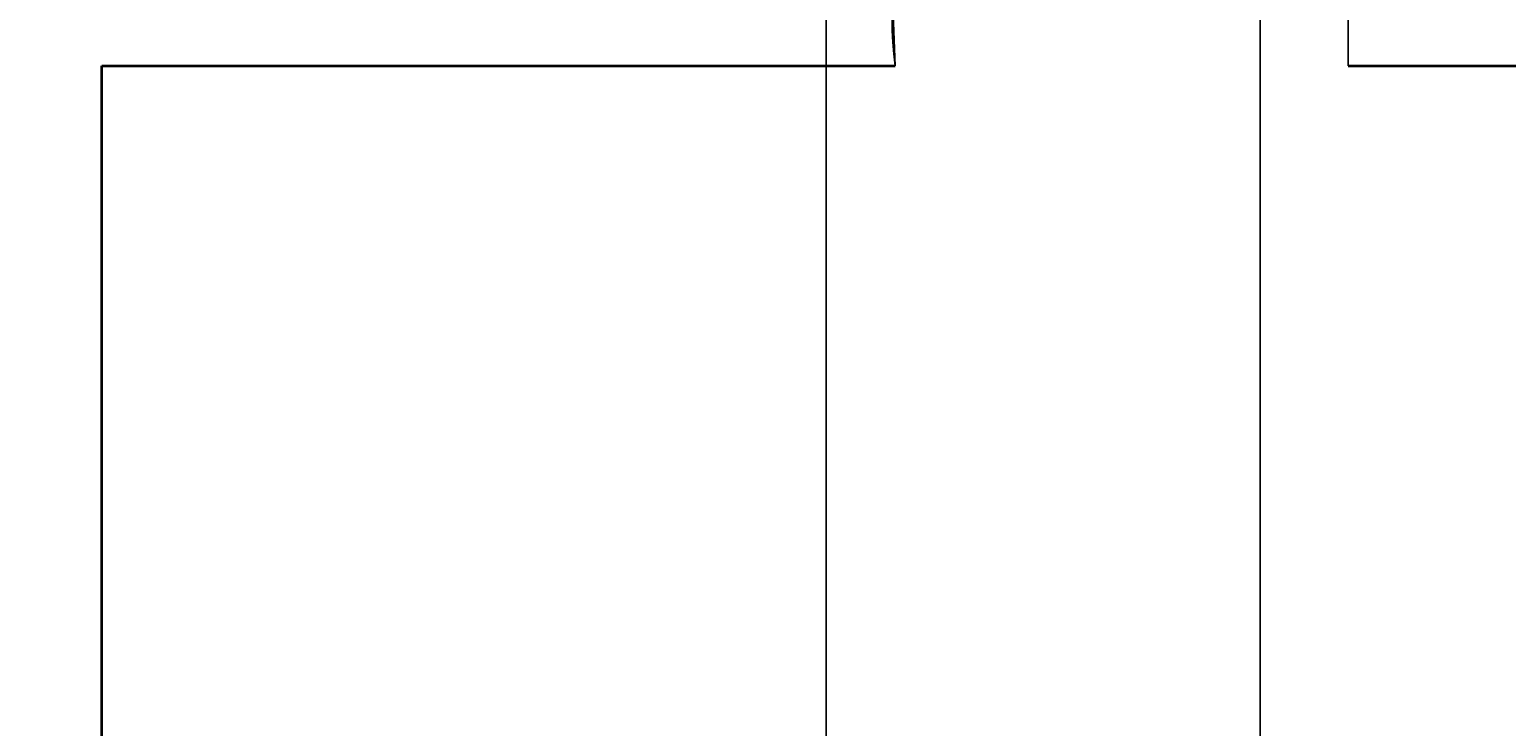
# Model space of a CAD drawing. Units: inches. Extents: x -61 to 1599, y -1316 to 257.
# Tile 111 of 204: x 114 to 236, y -68 to -10. Entities that reach past the tile are written whole.
import ezdxf

# ---------------------------------------------------------------- set-up
doc = ezdxf.new("R2010")
doc.units = ezdxf.units.IN
doc.header["$MEASUREMENT"] = 0
doc.linetypes.add('ACAD_ISO02W100', pattern=[15, 12, -3])
for name, color, linetype, lineweight in [('A-ANNO-DIMS', 2, 'Continuous', 18), ('A-WALL-JAMB', 4, 'ACAD_ISO02W100', 25), ('DOORS', 2, 'Continuous', 25), ('WALLS', 4, 'Continuous', 35)]:
    doc.layers.add(name, color=color, linetype=linetype, lineweight=lineweight)
doc.styles.get("Standard").update_dxf_attribs({"font": 'arial.ttf'})
doc.dimstyles.get("Standard").update_dxf_attribs({"dimtxt": 0.18, "dimasz": 0.18, "dimexe": 0.18, "dimexo": 0.0625, "dimgap": 0.09, "dimtad": 0, "dimtih": 1, "dimtoh": 1, "dimdec": 0, "dimzin": 0, "dimdsep": 46, "dimlunit": 3, "dimtxsty": 'Standard', "dimcen": 0.09, "dimadec": 0, "dimazin": 0, "dimtfac": 1, "dimtdec": 0, "dimtofl": 0, "dimtmove": 0, "dimatfit": 3, "dimfxl": 1, "dimtolj": 1, "dimtzin": 0, "dimarcsym": 0})

# ---------------------------------------------------------------- blocks, each defined once
blk = doc.blocks.new('DOOR-SWING-36')
blk.add_line((0, 0), (0, -5.4))
blk.add_lwpolyline([(0, 0), (0, 36), (-1.57, 36), (-1.57, 0)], close=True)
blk.add_arc((-0.74, -1.08), 37.09, 91.2913, 186.6905)
blk = doc.blocks.new('*D687')
at = {"layer": 'A-ANNO-DIMS', "color": 0, "lineweight": -2, "transparency": 16777216}
for p, q in [((289.42, 181.68), (-61.08, 181.68)), ((-60.9, 181.5), (-60.9, -528.95)), ((-60.9, -1239.76), (-60.9, -529.32)), ((319.64, -1239.94), (-61.08, -1239.94))]:
    blk.add_line(p, q, dxfattribs=at)
at = {"layer": 'A-ANNO-DIMS', "color": 0, "transparency": 16777216}
for points in [[(-60.93, 181.5), (-60.87, 181.5), (-60.9, 181.68)], [(-60.93, -1239.76), (-60.87, -1239.76), (-60.9, -1239.94)]]:
    blk.add_solid(points, dxfattribs=at)
at = {"layer": 'DEFPOINTS', "color": 0, "transparency": 16777216}
for p in [(289.48, 181.68), (-60.9, -1239.94), (319.7, -1239.94)]:
    blk.add_point(p, dxfattribs=at)
at = {"layer": 'A-ANNO-DIMS', "color": 0, "transparency": 16777216, "insert": (-60.9, -529.13), "char_height": 0.18, "attachment_point": 5}
blk.add_mtext('\\A1;1421.6', dxfattribs=at)
blk = doc.blocks.new('*D700')
at = {"layer": 'A-ANNO-DIMS', "color": 0, "lineweight": -2, "transparency": 16777216}
for p, q in [((14.7, -616.88), (14.7, 257.46)), ((14.88, 257.28), (96.77, 257.28)), ((179.57, 257.28), (97.68, 257.28)), ((179.75, -616.88), (179.75, 257.46))]:
    blk.add_line(p, q, dxfattribs=at)
at = {"layer": 'A-ANNO-DIMS', "color": 0, "transparency": 16777216}
for points in [[(14.88, 257.31), (14.88, 257.25), (14.7, 257.28)], [(179.57, 257.31), (179.57, 257.25), (179.75, 257.28)]]:
    blk.add_solid(points, dxfattribs=at)
at = {"layer": 'DEFPOINTS', "color": 0, "transparency": 16777216}
for p in [(179.75, 257.28), (14.7, -616.94), (179.75, -616.94)]:
    blk.add_point(p, dxfattribs=at)
at = {"layer": 'A-ANNO-DIMS', "color": 0, "transparency": 16777216, "insert": (97.23, 257.28), "char_height": 0.18, "attachment_point": 5}
blk.add_mtext('\\A1;165.05', dxfattribs=at)
blk = doc.blocks.new('*D701')
at = {"layer": 'A-ANNO-DIMS', "color": 0, "lineweight": -2, "transparency": 16777216}
for p, q in [((215.75, -616.88), (215.75, 257.46)), ((215.93, 257.28), (233.92, 257.28)), ((252.7, 257.28), (234.71, 257.28)), ((252.88, -616.88), (252.88, 257.46))]:
    blk.add_line(p, q, dxfattribs=at)
at = {"layer": 'A-ANNO-DIMS', "color": 0, "transparency": 16777216}
for points in [[(215.93, 257.31), (215.93, 257.25), (215.75, 257.28)], [(252.7, 257.31), (252.7, 257.25), (252.88, 257.28)]]:
    blk.add_solid(points, dxfattribs=at)
at = {"layer": 'DEFPOINTS', "color": 0, "transparency": 16777216}
for p in [(252.88, 257.28), (215.75, -616.94), (252.88, -616.94)]:
    blk.add_point(p, dxfattribs=at)
at = {"layer": 'A-ANNO-DIMS', "color": 0, "transparency": 16777216, "insert": (234.32, 257.28), "char_height": 0.18, "attachment_point": 5}
blk.add_mtext('\\A1;37.13', dxfattribs=at)

msp = doc.modelspace()

# ---------------------------------------------------------------- linework, layer by layer
at = {"layer": 'A-WALL-JAMB'}
for p, q in [((185.4756, -13.3229), (185.2611, -7.3229)), ((223.0506, -13.3229), (223.0506, -7.3229))]:
    msp.add_line(p, q, dxfattribs=at)
at = {"layer": 'WALLS'}
for p, q in [((119.7028, -169.3229), (119.7028, -13.3229)), ((119.7028, -13.3229), (185.4756, -13.3229)), ((223.0506, -13.3229), (237.7028, -13.3229))]:
    msp.add_line(p, q, dxfattribs=at)

# ---------------------------------------------------------------- block references
at = {"layer": 'DOORS'}
msp.add_blockref('DOOR-SWING-36', (223.0506, -7.9229), dxfattribs=at)

# ---------------------------------------------------------------- dimensions: what is measured, and where the dimension line sits
at = {"layer": 'A-ANNO-DIMS'}
for base, p1, p2, picture, middle in [((179.7521, 257.2771), (14.7028, -616.9446), (179.7521, -616.9446), '*D700', (97.2274, 257.2771)), ((252.8825, 257.2771), (215.7521, -616.9446), (252.8825, -616.9446), '*D701', (234.3173, 257.2771))]:
    dim = msp.add_linear_dim(base=base, p1=p1, p2=p2, dimstyle='Standard', override={"dimdec": 2, "dimlfac": 1, "dimrnd": 0, "dimzin": 0, "dimdsep": 46, "dimlunit": 2}, dxfattribs=at)
    dim.commit()
    dim.dimension.update_dxf_attribs({"geometry": picture, "text_midpoint": middle})
dim = msp.add_linear_dim(base=(-60.8972, -1239.9446), p1=(289.4807, 181.6771), p2=(319.7028, -1239.9446), angle=90, dimstyle='Standard', override={"dimdec": 1, "dimlfac": 1, "dimrnd": 0, "dimzin": 0, "dimdsep": 46, "dimlunit": 2}, dxfattribs=at)
dim.commit()
dim.dimension.update_dxf_attribs({"geometry": '*D687', "text_midpoint": (-60.8972, -529.1337)})

doc.saveas('drawing.dxf')
